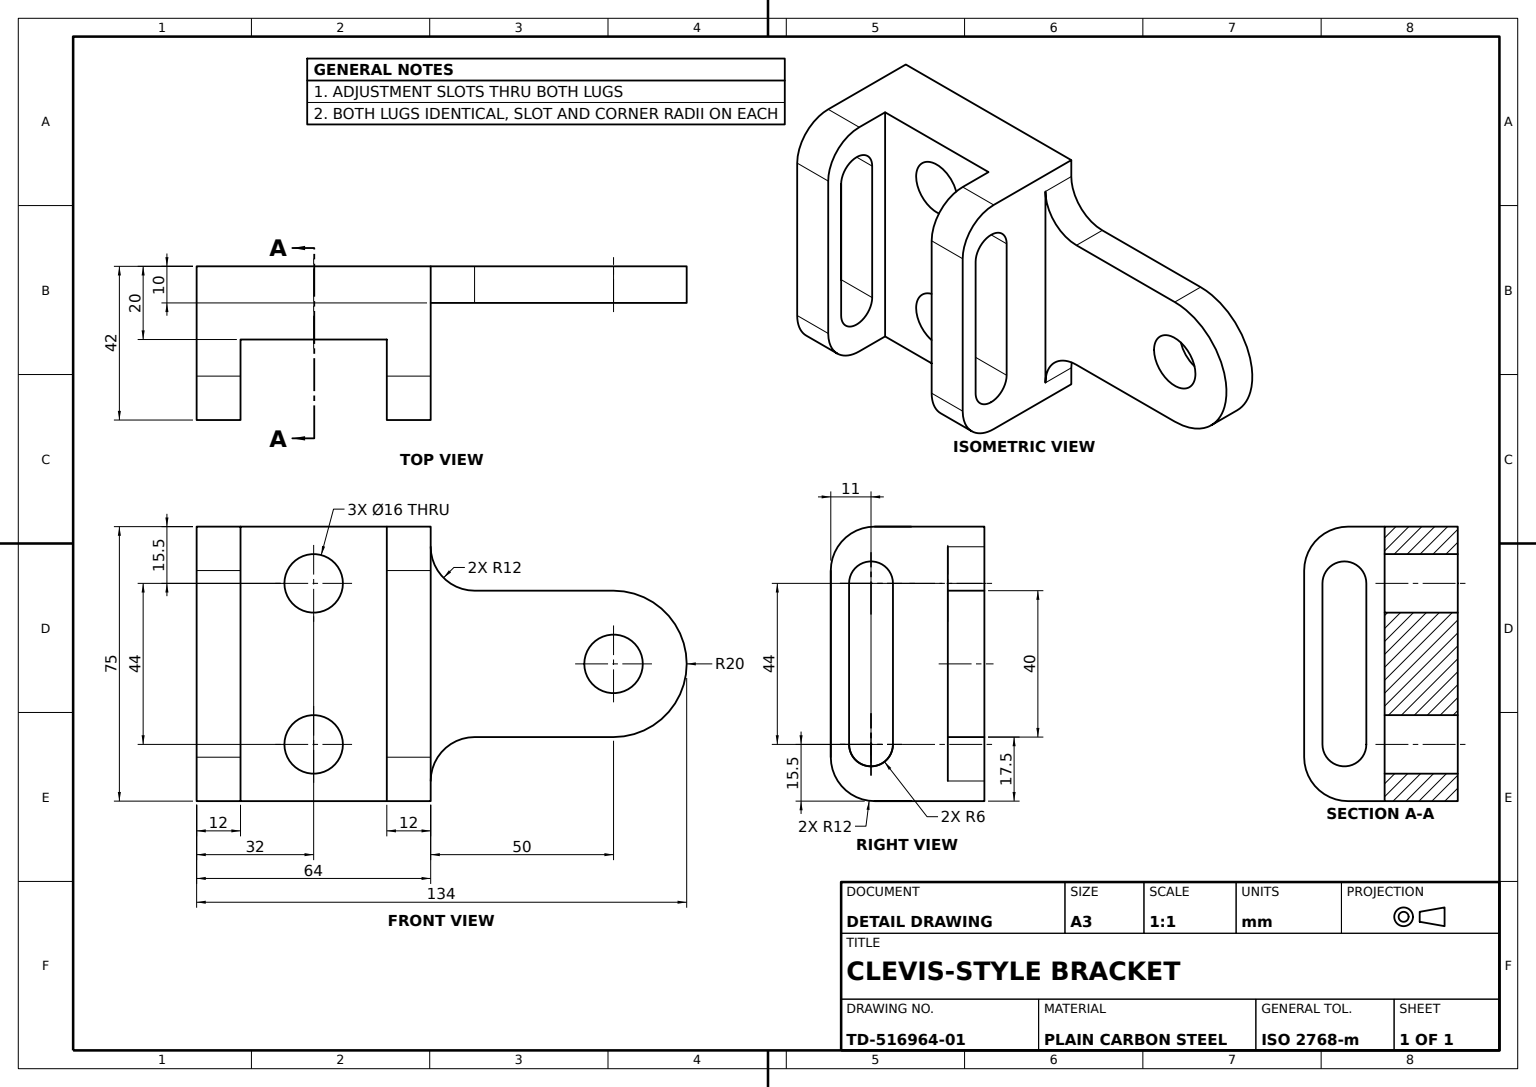
SolidWorks part; units mm, degrees
material "Plain Carbon Steel"
ref_plane "Front Plane" through (0, 0, 0) normal (0, 0, 1) x (1, 0, 0)
ref_plane "Top Plane" through (0, 0, 0) normal (0, 1, 0) x (1, 0, 0)
ref_plane "Right Plane" through (0, 0, 0) normal (1, 0, 0) x (0, 0, -1)
sketch "Base Block Sketch" plane through (0, 0, 0) normal (0, 0, 1) x (1, 0, 0)
  line L0 (0, 0) -> (64, 0)
  line L1 (64, 0) -> (64, 75)
  line L2 (64, 75) -> (0, 75)
  line L3 (0, 75) -> (0, 0)
  dimension "D1" = 64
  dimension "D2" = 75
extrude "Base Block" add sketch "Base Block Sketch" along normal blind 20
sketch "Clamp Lug A Sketch" plane through (0, 0, 20) normal (0, 0, 1) x (1, 0, 0)
  line L0 (0, 75) -> (0, 0) construction
  line L1 (0, 75) -> (12, 75)
  line L2 (0, 75) -> (0, 0)
  line L3 (0, 0) -> (12, 0)
  line L4 (12, 75) -> (12, 0)
  line L5 (64, 75) -> (0, 75) construction
  line L6 (0, 0) -> (64, 0) construction
  dimension "D1" = 12
extrude "Clamp Lug A" add sketch "Clamp Lug A Sketch" along normal blind 22
sketch "Clamp Lug B Sketch" plane through (0, 0, 20) normal (0, 0, 1) x (1, 0, 0)
  line L0 (64, 75) -> (12, 75) construction
  line L1 (52, 75) -> (64, 75)
  line L2 (52, 75) -> (52, 0)
  line L3 (52, 0) -> (64, 0)
  line L4 (64, 75) -> (64, 0)
  line L5 (12, 0) -> (64, 0) construction
  line L6 (64, 0) -> (64, 75) construction
  dimension "D1" = 12
extrude "Clamp Lug B" add sketch "Clamp Lug B Sketch" along normal blind 22
sketch "Adjustment Slot A Sketch" plane through (12, 0, 0) normal (1, 0, 0) x (0, 0, -1)
  line L0 (-31, 15.5) -> (-31, 59.5) construction
  line L1 (-37, 15.5) -> (-37, 59.5)
  line L2 (-25, 15.5) -> (-25, 59.5)
  line L3 (-42, 0) -> (-42, 75) construction
  arc A0 (-37, 15.5) -> (-25, 15.5) centre (-31, 15.5) ccw
  arc A1 (-25, 59.5) -> (-37, 59.5) centre (-31, 59.5) ccw
  point P2 (-31, 37.5)
  point P10 (-42, 37.5)
  dimension "D1" = 44
  dimension "D2" = 12
  dimension "D3" = 11
extrude "Adjustment Slot A" cut sketch "Adjustment Slot A Sketch" against normal through all
sketch "Adjustment Slot B Sketch" plane through (52, 0, 0) normal (-1, 0, 0) x (0, 0, 1)
  line L0 (31, 15.5) -> (31, 59.5) construction
  line L1 (25, 15.5) -> (25, 59.5)
  line L2 (37, 15.5) -> (37, 59.5)
  arc A0 (25, 15.5) -> (37, 15.5) centre (31, 15.5) ccw
  arc A1 (37, 59.5) -> (25, 59.5) centre (31, 59.5) ccw
  point P4 (31, 37.5)
  dimension "D1" = 6
extrude "Adjustment Slot B" cut sketch "Adjustment Slot B Sketch" against normal through all
ref_plane "Plane1" through (0, 0, 0) normal (0, 0, 1) x (1, 0, 0)
sketch "Mounting Tab Sketch" plane through (0, 0, 0) normal (0, 0, 1) x (1, 0, 0)
  line L0 (64, 0) -> (64, 75) construction
  line L1 (114, 57.5) -> (76, 57.5)
  line L2 (114, 17.5) -> (76, 17.5)
  line L3 (64, 69.5) -> (64, 5.5)
  circle A0 centre (114, 37.5) radius 8
  arc A1 (114, 17.5) -> (114, 57.5) centre (114, 37.5) ccw
  arc A2 (64, 69.5) -> (76, 57.5) centre (76, 69.5) ccw
  arc A3 (76, 17.5) -> (64, 5.5) centre (76, 5.5) ccw
  dimension "D1" = 16
  dimension "D2" = 40
  dimension "D4" = 24
  dimension "D5" = 24
  dimension "D3" = 50
  dimension "D6" = 37.5
extrude "Mounting Tab" add sketch "Mounting Tab Sketch" along normal blind 10
sketch "Back Wall Cut Sketch" plane through (0, 0, 20) normal (0, 0, 1) x (1, 0, 0)
  line L0 (12, 37.5) -> (32, 37.5) construction
  line L1 (12, 0) -> (12, 75) construction
  line L2 (52, 75) -> (52, 0) construction
  circle A0 centre (32, 59.5) radius 8
  circle A1 centre (32, 15.5) radius 8
  dimension "D1" = 16
  dimension "D2" = 16
  dimension "D3" = 22
  dimension "D4" = 22
  dimension "D5" = 20
extrude "Back Wall Cut" cut sketch "Back Wall Cut Sketch" against normal through all
fillet "Lug A Edge Fillet R12" radius 12 2 edges at (6, 0, 42) (6, 75, 42)
fillet "Lug B Edge Fillet R12" radius 12 2 edges at (58, 0, 42) (58, 75, 42)
